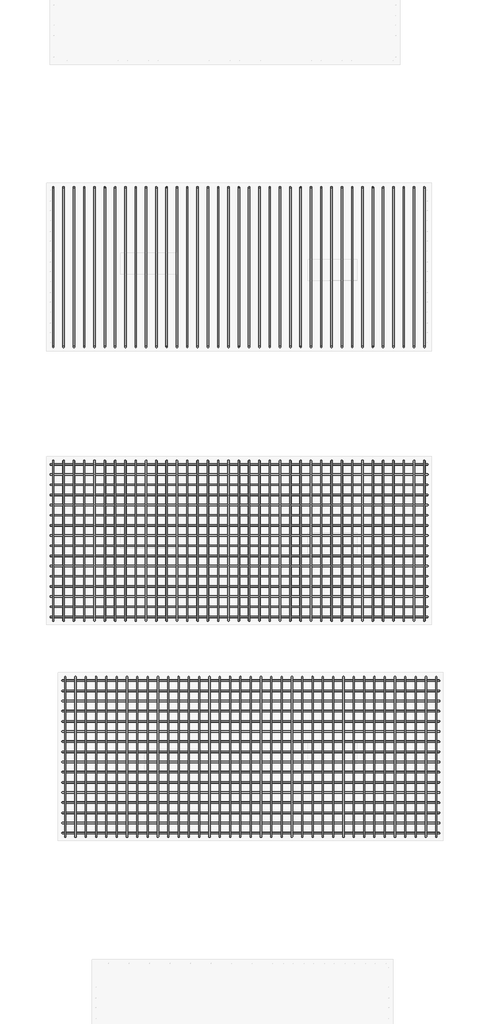
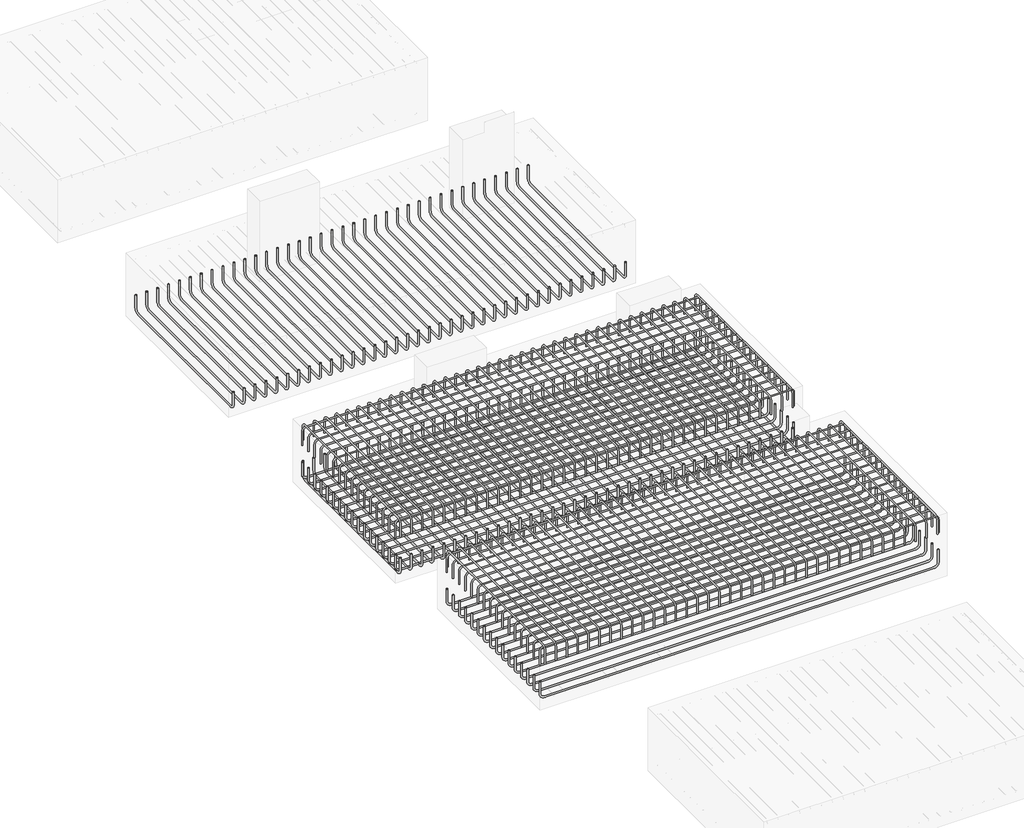
# One storey, part 5 of 21: 8 reinforcing bars.
"""IFC4 building model written with IfcOpenShell, lengths in millimetres."""

from ifc_helpers import new_model, si_unit, point, frame, origin, place, context, project, spatial, polyline, circle_curve, trimmed, segment, composite_curve, source, transform, mapped, element, save
from ifc_brep_helpers import swept_disk

model = new_model("IFC4")

# Units and contexts
model_context = context("Model", 3, world=origin())
ifc_project = project(units=[si_unit("LENGTHUNIT", "METRE", prefix="MILLI")], contexts=[model_context])

# Site, building, storey
site = spatial("IfcSite", under=ifc_project)
building = spatial("IfcBuilding", under=site)
storey = spatial("IfcBuildingStorey", under=building, Elevation=-1100.0)

# Reinforcing bars
placement = place(None, origin())
reinforcing_bar_shape = source(origin(), model_context, "Body", "SolidModel", [
    swept_disk(composite_curve([segment(polyline([(-19444.5839151, -8642.8795712, -1400.0), (-19444.5839151, -8642.8795712, -1213.4)]), True, "CONTINUOUS"), segment(trimmed(circle_curve(frame((-19444.5839151, -8587.4295712, -1213.4), z_axis=(-1.0, 0.0, 0.0), x_axis=(0.0, -55.44999999999891, 0.0)), 55.45), [point((-19444.5839151, -8642.8795712, -1213.4))], [point((-19444.5839151, -8587.4295712, -1157.95))], True, "CARTESIAN"), True, "CONTINUOUS"), segment(polyline([(-19444.5839151, -8587.4295712, -1157.95), (-19444.5839151, -6414.2295712, -1157.95)]), True, "CONTINUOUS"), segment(trimmed(circle_curve(frame((-19444.5839151, -6414.2295712, -1213.4), z_axis=(-1.0, 0.0, 0.0), x_axis=(0.0, 0.0, 55.450000000000045)), 55.45), [point((-19444.5839151, -6414.2295712, -1157.95))], [point((-19444.5839151, -6358.7795712, -1213.4))], True, "CARTESIAN"), True, "CONTINUOUS"), segment(polyline([(-19444.5839151, -6358.7795712, -1213.4), (-19444.5839151, -6358.7795712, -1400.0)]), True, "CONTINUOUS")], self_intersect=False), 7.95),
])
element("IfcReinforcingBar", 1, at=placement, inside=storey, context=model_context, shape_type="MappedRepresentation", body=[
    mapped(reinforcing_bar_shape, transform((0.0, 0.0, 0.0), x_axis=(1.0, 0.0, 0.0), y_axis=(0.0, 1.0, 0.0), z_axis=(0.0, 0.0, 1.0))),
    mapped(reinforcing_bar_shape, transform((147.2696553, 0.0, 0.0), x_axis=(1.0, 0.0, 0.0), y_axis=(0.0, 1.0, 0.0), z_axis=(0.0, 0.0, 1.0))),
    mapped(reinforcing_bar_shape, transform((294.5393106, 0.0, 0.0), x_axis=(1.0, 0.0, 0.0), y_axis=(0.0, 1.0, 0.0), z_axis=(0.0, 0.0, 1.0))),
    mapped(reinforcing_bar_shape, transform((441.8089659, 0.0, 0.0), x_axis=(1.0, 0.0, 0.0), y_axis=(0.0, 1.0, 0.0), z_axis=(0.0, 0.0, 1.0))),
    mapped(reinforcing_bar_shape, transform((589.0786213, 0.0, 0.0), x_axis=(1.0, 0.0, 0.0), y_axis=(0.0, 1.0, 0.0), z_axis=(0.0, 0.0, 1.0))),
    mapped(reinforcing_bar_shape, transform((736.3482766, 0.0, 0.0), x_axis=(1.0, 0.0, 0.0), y_axis=(0.0, 1.0, 0.0), z_axis=(0.0, 0.0, 1.0))),
    mapped(reinforcing_bar_shape, transform((883.6179319, 0.0, 0.0), x_axis=(1.0, 0.0, 0.0), y_axis=(0.0, 1.0, 0.0), z_axis=(0.0, 0.0, 1.0))),
    mapped(reinforcing_bar_shape, transform((1030.8875872, 0.0, 0.0), x_axis=(1.0, 0.0, 0.0), y_axis=(0.0, 1.0, 0.0), z_axis=(0.0, 0.0, 1.0))),
    mapped(reinforcing_bar_shape, transform((1178.1572425, 0.0, 0.0), x_axis=(1.0, 0.0, 0.0), y_axis=(0.0, 1.0, 0.0), z_axis=(0.0, 0.0, 1.0))),
    mapped(reinforcing_bar_shape, transform((1325.4268978, 0.0, 0.0), x_axis=(1.0, 0.0, 0.0), y_axis=(0.0, 1.0, 0.0), z_axis=(0.0, 0.0, 1.0))),
    mapped(reinforcing_bar_shape, transform((1472.6965532, 0.0, 0.0), x_axis=(1.0, 0.0, 0.0), y_axis=(0.0, 1.0, 0.0), z_axis=(0.0, 0.0, 1.0))),
    mapped(reinforcing_bar_shape, transform((1619.9662085, 0.0, 0.0), x_axis=(1.0, 0.0, 0.0), y_axis=(0.0, 1.0, 0.0), z_axis=(0.0, 0.0, 1.0))),
    mapped(reinforcing_bar_shape, transform((1767.2358638, 0.0, 0.0), x_axis=(1.0, 0.0, 0.0), y_axis=(0.0, 1.0, 0.0), z_axis=(0.0, 0.0, 1.0))),
    mapped(reinforcing_bar_shape, transform((1914.5055191, 0.0, 0.0), x_axis=(1.0, 0.0, 0.0), y_axis=(0.0, 1.0, 0.0), z_axis=(0.0, 0.0, 1.0))),
    mapped(reinforcing_bar_shape, transform((2061.7751744, 0.0, 0.0), x_axis=(1.0, 0.0, 0.0), y_axis=(0.0, 1.0, 0.0), z_axis=(0.0, 0.0, 1.0))),
    mapped(reinforcing_bar_shape, transform((2209.0448297, 0.0, 0.0), x_axis=(1.0, 0.0, 0.0), y_axis=(0.0, 1.0, 0.0), z_axis=(0.0, 0.0, 1.0))),
    mapped(reinforcing_bar_shape, transform((2356.314485, 0.0, 0.0), x_axis=(1.0, 0.0, 0.0), y_axis=(0.0, 1.0, 0.0), z_axis=(0.0, 0.0, 1.0))),
    mapped(reinforcing_bar_shape, transform((2503.5841404, 0.0, 0.0), x_axis=(1.0, 0.0, 0.0), y_axis=(0.0, 1.0, 0.0), z_axis=(0.0, 0.0, 1.0))),
    mapped(reinforcing_bar_shape, transform((2650.8537957, 0.0, 0.0), x_axis=(1.0, 0.0, 0.0), y_axis=(0.0, 1.0, 0.0), z_axis=(0.0, 0.0, 1.0))),
    mapped(reinforcing_bar_shape, transform((2798.123451, 0.0, 0.0), x_axis=(1.0, 0.0, 0.0), y_axis=(0.0, 1.0, 0.0), z_axis=(0.0, 0.0, 1.0))),
    mapped(reinforcing_bar_shape, transform((2945.3931063, 0.0, 0.0), x_axis=(1.0, 0.0, 0.0), y_axis=(0.0, 1.0, 0.0), z_axis=(0.0, 0.0, 1.0))),
    mapped(reinforcing_bar_shape, transform((3092.6627616, 0.0, 0.0), x_axis=(1.0, 0.0, 0.0), y_axis=(0.0, 1.0, 0.0), z_axis=(0.0, 0.0, 1.0))),
    mapped(reinforcing_bar_shape, transform((3239.9324169, 0.0, 0.0), x_axis=(1.0, 0.0, 0.0), y_axis=(0.0, 1.0, 0.0), z_axis=(0.0, 0.0, 1.0))),
    mapped(reinforcing_bar_shape, transform((3387.2020722, 0.0, 0.0), x_axis=(1.0, 0.0, 0.0), y_axis=(0.0, 1.0, 0.0), z_axis=(0.0, 0.0, 1.0))),
    mapped(reinforcing_bar_shape, transform((3534.4717276, 0.0, 0.0), x_axis=(1.0, 0.0, 0.0), y_axis=(0.0, 1.0, 0.0), z_axis=(0.0, 0.0, 1.0))),
    mapped(reinforcing_bar_shape, transform((3681.7413829, 0.0, 0.0), x_axis=(1.0, 0.0, 0.0), y_axis=(0.0, 1.0, 0.0), z_axis=(0.0, 0.0, 1.0))),
    mapped(reinforcing_bar_shape, transform((3829.0110382, 0.0, 0.0), x_axis=(1.0, 0.0, 0.0), y_axis=(0.0, 1.0, 0.0), z_axis=(0.0, 0.0, 1.0))),
    mapped(reinforcing_bar_shape, transform((3976.2806935, 0.0, 0.0), x_axis=(1.0, 0.0, 0.0), y_axis=(0.0, 1.0, 0.0), z_axis=(0.0, 0.0, 1.0))),
    mapped(reinforcing_bar_shape, transform((4123.5503488, 0.0, 0.0), x_axis=(1.0, 0.0, 0.0), y_axis=(0.0, 1.0, 0.0), z_axis=(0.0, 0.0, 1.0))),
    mapped(reinforcing_bar_shape, transform((4270.8200041, 0.0, 0.0), x_axis=(1.0, 0.0, 0.0), y_axis=(0.0, 1.0, 0.0), z_axis=(0.0, 0.0, 1.0))),
    mapped(reinforcing_bar_shape, transform((4418.0896595, 0.0, 0.0), x_axis=(1.0, 0.0, 0.0), y_axis=(0.0, 1.0, 0.0), z_axis=(0.0, 0.0, 1.0))),
    mapped(reinforcing_bar_shape, transform((4565.3593148, 0.0, 0.0), x_axis=(1.0, 0.0, 0.0), y_axis=(0.0, 1.0, 0.0), z_axis=(0.0, 0.0, 1.0))),
    mapped(reinforcing_bar_shape, transform((4712.6289701, 0.0, 0.0), x_axis=(1.0, 0.0, 0.0), y_axis=(0.0, 1.0, 0.0), z_axis=(0.0, 0.0, 1.0))),
    mapped(reinforcing_bar_shape, transform((4859.8986254, 0.0, 0.0), x_axis=(1.0, 0.0, 0.0), y_axis=(0.0, 1.0, 0.0), z_axis=(0.0, 0.0, 1.0))),
    mapped(reinforcing_bar_shape, transform((5007.1682807, 0.0, 0.0), x_axis=(1.0, 0.0, 0.0), y_axis=(0.0, 1.0, 0.0), z_axis=(0.0, 0.0, 1.0))),
    mapped(reinforcing_bar_shape, transform((5154.437936, 0.0, 0.0), x_axis=(1.0, 0.0, 0.0), y_axis=(0.0, 1.0, 0.0), z_axis=(0.0, 0.0, 1.0))),
    mapped(reinforcing_bar_shape, transform((5301.7075913, 0.0, 0.0), x_axis=(1.0, 0.0, 0.0), y_axis=(0.0, 1.0, 0.0), z_axis=(0.0, 0.0, 1.0))),
])
reinforcing_bar_2_shape = source(origin(), model_context, "Body", "SolidModel", [
    swept_disk(composite_curve([segment(polyline([(-19482.8826863, -6410.6137352, -1428.1111113), (-19482.8826863, -6410.6137352, -1241.5111113)]), True, "CONTINUOUS"), segment(trimmed(circle_curve(frame((-19427.4326863, -6410.6137352, -1241.5111113), z_axis=(0.0, 1.0, 0.0), x_axis=(-55.45000000000073, 0.0, 0.0)), 55.45), [point((-19482.8826863, -6410.6137352, -1241.5111113))], [point((-19427.4326863, -6410.6137352, -1186.0611113))], True, "CARTESIAN"), True, "CONTINUOUS"), segment(polyline([(-19427.4326863, -6410.6137352, -1186.0611113), (-14154.2326863, -6410.6137352, -1186.0611113)]), True, "CONTINUOUS"), segment(trimmed(circle_curve(frame((-14154.2326863, -6410.6137352, -1241.5111113), z_axis=(0.0, 1.0, 0.0), x_axis=(0.0, 0.0, 55.450000000000045)), 55.45), [point((-14154.2326863, -6410.6137352, -1186.0611113))], [point((-14098.7826863, -6410.6137352, -1241.5111113))], True, "CARTESIAN"), True, "CONTINUOUS"), segment(polyline([(-14098.7826863, -6410.6137352, -1241.5111113), (-14098.7826863, -6410.6137352, -1428.1111113)]), True, "CONTINUOUS")], self_intersect=False), 7.95),
])
element("IfcReinforcingBar", 2, at=placement, inside=storey, context=model_context, shape_type="MappedRepresentation", body=[
    mapped(reinforcing_bar_2_shape, transform((0.0, 0.0, 0.0), x_axis=(1.0, 0.0, 0.0), y_axis=(0.0, 1.0, 0.0), z_axis=(0.0, 0.0, 1.0))),
    mapped(reinforcing_bar_2_shape, transform((0.0, -145.2528929, 0.0), x_axis=(1.0, 0.0, 0.0), y_axis=(0.0, 1.0, 0.0), z_axis=(0.0, 0.0, 1.0))),
    mapped(reinforcing_bar_2_shape, transform((0.0, -290.5057858, 0.0), x_axis=(1.0, 0.0, 0.0), y_axis=(0.0, 1.0, 0.0), z_axis=(0.0, 0.0, 1.0))),
    mapped(reinforcing_bar_2_shape, transform((0.0, -435.7586787, 0.0), x_axis=(1.0, 0.0, 0.0), y_axis=(0.0, 1.0, 0.0), z_axis=(0.0, 0.0, 1.0))),
    mapped(reinforcing_bar_2_shape, transform((0.0, -581.0115716, 0.0), x_axis=(1.0, 0.0, 0.0), y_axis=(0.0, 1.0, 0.0), z_axis=(0.0, 0.0, 1.0))),
    mapped(reinforcing_bar_2_shape, transform((0.0, -726.2644645, 0.0), x_axis=(1.0, 0.0, 0.0), y_axis=(0.0, 1.0, 0.0), z_axis=(0.0, 0.0, 1.0))),
    mapped(reinforcing_bar_2_shape, transform((0.0, -871.5173574, 0.0), x_axis=(1.0, 0.0, 0.0), y_axis=(0.0, 1.0, 0.0), z_axis=(0.0, 0.0, 1.0))),
    mapped(reinforcing_bar_2_shape, transform((0.0, -1016.7702503, 0.0), x_axis=(1.0, 0.0, 0.0), y_axis=(0.0, 1.0, 0.0), z_axis=(0.0, 0.0, 1.0))),
    mapped(reinforcing_bar_2_shape, transform((0.0, -1162.0231432, 0.0), x_axis=(1.0, 0.0, 0.0), y_axis=(0.0, 1.0, 0.0), z_axis=(0.0, 0.0, 1.0))),
    mapped(reinforcing_bar_2_shape, transform((0.0, -1307.276036, 0.0), x_axis=(1.0, 0.0, 0.0), y_axis=(0.0, 1.0, 0.0), z_axis=(0.0, 0.0, 1.0))),
    mapped(reinforcing_bar_2_shape, transform((0.0, -1452.5289289, 0.0), x_axis=(1.0, 0.0, 0.0), y_axis=(0.0, 1.0, 0.0), z_axis=(0.0, 0.0, 1.0))),
    mapped(reinforcing_bar_2_shape, transform((0.0, -1597.7818218, 0.0), x_axis=(1.0, 0.0, 0.0), y_axis=(0.0, 1.0, 0.0), z_axis=(0.0, 0.0, 1.0))),
    mapped(reinforcing_bar_2_shape, transform((0.0, -1743.0347147, 0.0), x_axis=(1.0, 0.0, 0.0), y_axis=(0.0, 1.0, 0.0), z_axis=(0.0, 0.0, 1.0))),
    mapped(reinforcing_bar_2_shape, transform((0.0, -1888.2876076, 0.0), x_axis=(1.0, 0.0, 0.0), y_axis=(0.0, 1.0, 0.0), z_axis=(0.0, 0.0, 1.0))),
    mapped(reinforcing_bar_2_shape, transform((0.0, -2033.5405005, 0.0), x_axis=(1.0, 0.0, 0.0), y_axis=(0.0, 1.0, 0.0), z_axis=(0.0, 0.0, 1.0))),
    mapped(reinforcing_bar_2_shape, transform((0.0, -2178.7933934, 0.0), x_axis=(1.0, 0.0, 0.0), y_axis=(0.0, 1.0, 0.0), z_axis=(0.0, 0.0, 1.0))),
])
reinforcing_bar_3_shape = source(origin(), model_context, "Body", "SolidModel", [
    swept_disk(composite_curve([segment(polyline([(-19480.8326863, -8589.4071286, -1669.8442859), (-19480.8326863, -8589.4071286, -1852.3442859)]), True, "CONTINUOUS"), segment(trimmed(circle_curve(frame((-19423.3326863, -8589.4071286, -1852.3442859), z_axis=(0.0, -1.0, 0.0), x_axis=(-57.5, 0.0, 0.0)), 57.5), [point((-19480.8326863, -8589.4071286, -1852.3442859))], [point((-19423.3326863, -8589.4071286, -1909.8442859))], True, "CARTESIAN"), True, "CONTINUOUS"), segment(polyline([(-19423.3326863, -8589.4071286, -1909.8442859), (-14158.3326863, -8589.4071286, -1909.8442859)]), True, "CONTINUOUS"), segment(trimmed(circle_curve(frame((-14158.3326863, -8589.4071286, -1852.3442859), z_axis=(0.0, -1.0, 0.0), x_axis=(0.0, 0.0, -57.5)), 57.5), [point((-14158.3326863, -8589.4071286, -1909.8442859))], [point((-14100.8326863, -8589.4071286, -1852.3442859))], True, "CARTESIAN"), True, "CONTINUOUS"), segment(polyline([(-14100.8326863, -8589.4071286, -1852.3442859), (-14100.8326863, -8589.4071286, -1669.8442859)]), True, "CONTINUOUS")], self_intersect=False), 10.0),
])
element("IfcReinforcingBar", 3, at=placement, inside=storey, context=model_context, shape_type="MappedRepresentation", body=[
    mapped(reinforcing_bar_3_shape, transform((0.0, 0.0, 0.0), x_axis=(1.0, 0.0, 0.0), y_axis=(0.0, 1.0, 0.0), z_axis=(0.0, 0.0, 1.0))),
    mapped(reinforcing_bar_3_shape, transform((0.0, 145.2528929, 0.0), x_axis=(1.0, 0.0, 0.0), y_axis=(0.0, 1.0, 0.0), z_axis=(0.0, 0.0, 1.0))),
    mapped(reinforcing_bar_3_shape, transform((0.0, 290.5057858, 0.0), x_axis=(1.0, 0.0, 0.0), y_axis=(0.0, 1.0, 0.0), z_axis=(0.0, 0.0, 1.0))),
    mapped(reinforcing_bar_3_shape, transform((0.0, 435.7586787, 0.0), x_axis=(1.0, 0.0, 0.0), y_axis=(0.0, 1.0, 0.0), z_axis=(0.0, 0.0, 1.0))),
    mapped(reinforcing_bar_3_shape, transform((0.0, 581.0115716, 0.0), x_axis=(1.0, 0.0, 0.0), y_axis=(0.0, 1.0, 0.0), z_axis=(0.0, 0.0, 1.0))),
    mapped(reinforcing_bar_3_shape, transform((0.0, 726.2644645, 0.0), x_axis=(1.0, 0.0, 0.0), y_axis=(0.0, 1.0, 0.0), z_axis=(0.0, 0.0, 1.0))),
    mapped(reinforcing_bar_3_shape, transform((0.0, 871.5173574, 0.0), x_axis=(1.0, 0.0, 0.0), y_axis=(0.0, 1.0, 0.0), z_axis=(0.0, 0.0, 1.0))),
    mapped(reinforcing_bar_3_shape, transform((0.0, 1016.7702503, 0.0), x_axis=(1.0, 0.0, 0.0), y_axis=(0.0, 1.0, 0.0), z_axis=(0.0, 0.0, 1.0))),
    mapped(reinforcing_bar_3_shape, transform((0.0, 1162.0231432, 0.0), x_axis=(1.0, 0.0, 0.0), y_axis=(0.0, 1.0, 0.0), z_axis=(0.0, 0.0, 1.0))),
    mapped(reinforcing_bar_3_shape, transform((0.0, 1307.276036, 0.0), x_axis=(1.0, 0.0, 0.0), y_axis=(0.0, 1.0, 0.0), z_axis=(0.0, 0.0, 1.0))),
    mapped(reinforcing_bar_3_shape, transform((0.0, 1452.5289289, 0.0), x_axis=(1.0, 0.0, 0.0), y_axis=(0.0, 1.0, 0.0), z_axis=(0.0, 0.0, 1.0))),
    mapped(reinforcing_bar_3_shape, transform((0.0, 1597.7818218, 0.0), x_axis=(1.0, 0.0, 0.0), y_axis=(0.0, 1.0, 0.0), z_axis=(0.0, 0.0, 1.0))),
    mapped(reinforcing_bar_3_shape, transform((0.0, 1743.0347147, 0.0), x_axis=(1.0, 0.0, 0.0), y_axis=(0.0, 1.0, 0.0), z_axis=(0.0, 0.0, 1.0))),
    mapped(reinforcing_bar_3_shape, transform((0.0, 1888.2876076, 0.0), x_axis=(1.0, 0.0, 0.0), y_axis=(0.0, 1.0, 0.0), z_axis=(0.0, 0.0, 1.0))),
    mapped(reinforcing_bar_3_shape, transform((0.0, 2033.5405005, 0.0), x_axis=(1.0, 0.0, 0.0), y_axis=(0.0, 1.0, 0.0), z_axis=(0.0, 0.0, 1.0))),
    mapped(reinforcing_bar_3_shape, transform((0.0, 2178.7933934, 0.0), x_axis=(1.0, 0.0, 0.0), y_axis=(0.0, 1.0, 0.0), z_axis=(0.0, 0.0, 1.0))),
])
reinforcing_bar_4_shape = source(origin(), model_context, "Body", "SolidModel", [
    swept_disk(composite_curve([segment(polyline([(-19614.5839151, -3270.8295712, -1700.0), (-19614.5839151, -3270.8295712, -1882.5)]), True, "CONTINUOUS"), segment(trimmed(circle_curve(frame((-19614.5839151, -3328.3295712, -1882.5), z_axis=(-1.0, 0.0, 0.0), x_axis=(0.0, 57.5, 0.0)), 57.5), [point((-19614.5839151, -3270.8295712, -1882.5))], [point((-19614.5839151, -3328.3295712, -1940.0))], True, "CARTESIAN"), True, "CONTINUOUS"), segment(polyline([(-19614.5839151, -3328.3295712, -1940.0), (-19614.5839151, -5493.3295712, -1940.0)]), True, "CONTINUOUS"), segment(trimmed(circle_curve(frame((-19614.5839151, -5493.3295712, -1882.5), z_axis=(-1.0, 0.0, 0.0), x_axis=(0.0, 0.0, -57.5)), 57.5), [point((-19614.5839151, -5493.3295712, -1940.0))], [point((-19614.5839151, -5550.8295712, -1882.5))], True, "CARTESIAN"), True, "CONTINUOUS"), segment(polyline([(-19614.5839151, -5550.8295712, -1882.5), (-19614.5839151, -5550.8295712, -1700.0)]), True, "CONTINUOUS")], self_intersect=False), 10.0),
])
element("IfcReinforcingBar", 4, at=placement, inside=storey, context=model_context, shape_type="MappedRepresentation", body=[
    mapped(reinforcing_bar_4_shape, transform((0.0, 0.0, 0.0), x_axis=(1.0, 0.0, 0.0), y_axis=(0.0, 1.0, 0.0), z_axis=(0.0, 0.0, 1.0))),
    mapped(reinforcing_bar_4_shape, transform((147.2696553, 0.0, 0.0), x_axis=(1.0, 0.0, 0.0), y_axis=(0.0, 1.0, 0.0), z_axis=(0.0, 0.0, 1.0))),
    mapped(reinforcing_bar_4_shape, transform((294.5393106, 0.0, 0.0), x_axis=(1.0, 0.0, 0.0), y_axis=(0.0, 1.0, 0.0), z_axis=(0.0, 0.0, 1.0))),
    mapped(reinforcing_bar_4_shape, transform((441.8089659, 0.0, 0.0), x_axis=(1.0, 0.0, 0.0), y_axis=(0.0, 1.0, 0.0), z_axis=(0.0, 0.0, 1.0))),
    mapped(reinforcing_bar_4_shape, transform((589.0786213, 0.0, 0.0), x_axis=(1.0, 0.0, 0.0), y_axis=(0.0, 1.0, 0.0), z_axis=(0.0, 0.0, 1.0))),
    mapped(reinforcing_bar_4_shape, transform((736.3482766, 0.0, 0.0), x_axis=(1.0, 0.0, 0.0), y_axis=(0.0, 1.0, 0.0), z_axis=(0.0, 0.0, 1.0))),
    mapped(reinforcing_bar_4_shape, transform((883.6179319, 0.0, 0.0), x_axis=(1.0, 0.0, 0.0), y_axis=(0.0, 1.0, 0.0), z_axis=(0.0, 0.0, 1.0))),
    mapped(reinforcing_bar_4_shape, transform((1030.8875872, 0.0, 0.0), x_axis=(1.0, 0.0, 0.0), y_axis=(0.0, 1.0, 0.0), z_axis=(0.0, 0.0, 1.0))),
    mapped(reinforcing_bar_4_shape, transform((1178.1572425, 0.0, 0.0), x_axis=(1.0, 0.0, 0.0), y_axis=(0.0, 1.0, 0.0), z_axis=(0.0, 0.0, 1.0))),
    mapped(reinforcing_bar_4_shape, transform((1325.4268978, 0.0, 0.0), x_axis=(1.0, 0.0, 0.0), y_axis=(0.0, 1.0, 0.0), z_axis=(0.0, 0.0, 1.0))),
    mapped(reinforcing_bar_4_shape, transform((1472.6965532, 0.0, 0.0), x_axis=(1.0, 0.0, 0.0), y_axis=(0.0, 1.0, 0.0), z_axis=(0.0, 0.0, 1.0))),
    mapped(reinforcing_bar_4_shape, transform((1619.9662085, 0.0, 0.0), x_axis=(1.0, 0.0, 0.0), y_axis=(0.0, 1.0, 0.0), z_axis=(0.0, 0.0, 1.0))),
    mapped(reinforcing_bar_4_shape, transform((1767.2358638, 0.0, 0.0), x_axis=(1.0, 0.0, 0.0), y_axis=(0.0, 1.0, 0.0), z_axis=(0.0, 0.0, 1.0))),
    mapped(reinforcing_bar_4_shape, transform((1914.5055191, 0.0, 0.0), x_axis=(1.0, 0.0, 0.0), y_axis=(0.0, 1.0, 0.0), z_axis=(0.0, 0.0, 1.0))),
    mapped(reinforcing_bar_4_shape, transform((2061.7751744, 0.0, 0.0), x_axis=(1.0, 0.0, 0.0), y_axis=(0.0, 1.0, 0.0), z_axis=(0.0, 0.0, 1.0))),
    mapped(reinforcing_bar_4_shape, transform((2209.0448297, 0.0, 0.0), x_axis=(1.0, 0.0, 0.0), y_axis=(0.0, 1.0, 0.0), z_axis=(0.0, 0.0, 1.0))),
    mapped(reinforcing_bar_4_shape, transform((2356.314485, 0.0, 0.0), x_axis=(1.0, 0.0, 0.0), y_axis=(0.0, 1.0, 0.0), z_axis=(0.0, 0.0, 1.0))),
    mapped(reinforcing_bar_4_shape, transform((2503.5841404, 0.0, 0.0), x_axis=(1.0, 0.0, 0.0), y_axis=(0.0, 1.0, 0.0), z_axis=(0.0, 0.0, 1.0))),
    mapped(reinforcing_bar_4_shape, transform((2650.8537957, 0.0, 0.0), x_axis=(1.0, 0.0, 0.0), y_axis=(0.0, 1.0, 0.0), z_axis=(0.0, 0.0, 1.0))),
    mapped(reinforcing_bar_4_shape, transform((2798.123451, 0.0, 0.0), x_axis=(1.0, 0.0, 0.0), y_axis=(0.0, 1.0, 0.0), z_axis=(0.0, 0.0, 1.0))),
    mapped(reinforcing_bar_4_shape, transform((2945.3931063, 0.0, 0.0), x_axis=(1.0, 0.0, 0.0), y_axis=(0.0, 1.0, 0.0), z_axis=(0.0, 0.0, 1.0))),
    mapped(reinforcing_bar_4_shape, transform((3092.6627616, 0.0, 0.0), x_axis=(1.0, 0.0, 0.0), y_axis=(0.0, 1.0, 0.0), z_axis=(0.0, 0.0, 1.0))),
    mapped(reinforcing_bar_4_shape, transform((3239.9324169, 0.0, 0.0), x_axis=(1.0, 0.0, 0.0), y_axis=(0.0, 1.0, 0.0), z_axis=(0.0, 0.0, 1.0))),
    mapped(reinforcing_bar_4_shape, transform((3387.2020722, 0.0, 0.0), x_axis=(1.0, 0.0, 0.0), y_axis=(0.0, 1.0, 0.0), z_axis=(0.0, 0.0, 1.0))),
    mapped(reinforcing_bar_4_shape, transform((3534.4717276, 0.0, 0.0), x_axis=(1.0, 0.0, 0.0), y_axis=(0.0, 1.0, 0.0), z_axis=(0.0, 0.0, 1.0))),
    mapped(reinforcing_bar_4_shape, transform((3681.7413829, 0.0, 0.0), x_axis=(1.0, 0.0, 0.0), y_axis=(0.0, 1.0, 0.0), z_axis=(0.0, 0.0, 1.0))),
    mapped(reinforcing_bar_4_shape, transform((3829.0110382, 0.0, 0.0), x_axis=(1.0, 0.0, 0.0), y_axis=(0.0, 1.0, 0.0), z_axis=(0.0, 0.0, 1.0))),
    mapped(reinforcing_bar_4_shape, transform((3976.2806935, 0.0, 0.0), x_axis=(1.0, 0.0, 0.0), y_axis=(0.0, 1.0, 0.0), z_axis=(0.0, 0.0, 1.0))),
    mapped(reinforcing_bar_4_shape, transform((4123.5503488, 0.0, 0.0), x_axis=(1.0, 0.0, 0.0), y_axis=(0.0, 1.0, 0.0), z_axis=(0.0, 0.0, 1.0))),
    mapped(reinforcing_bar_4_shape, transform((4270.8200041, 0.0, 0.0), x_axis=(1.0, 0.0, 0.0), y_axis=(0.0, 1.0, 0.0), z_axis=(0.0, 0.0, 1.0))),
    mapped(reinforcing_bar_4_shape, transform((4418.0896595, 0.0, 0.0), x_axis=(1.0, 0.0, 0.0), y_axis=(0.0, 1.0, 0.0), z_axis=(0.0, 0.0, 1.0))),
    mapped(reinforcing_bar_4_shape, transform((4565.3593148, 0.0, 0.0), x_axis=(1.0, 0.0, 0.0), y_axis=(0.0, 1.0, 0.0), z_axis=(0.0, 0.0, 1.0))),
    mapped(reinforcing_bar_4_shape, transform((4712.6289701, 0.0, 0.0), x_axis=(1.0, 0.0, 0.0), y_axis=(0.0, 1.0, 0.0), z_axis=(0.0, 0.0, 1.0))),
    mapped(reinforcing_bar_4_shape, transform((4859.8986254, 0.0, 0.0), x_axis=(1.0, 0.0, 0.0), y_axis=(0.0, 1.0, 0.0), z_axis=(0.0, 0.0, 1.0))),
    mapped(reinforcing_bar_4_shape, transform((5007.1682807, 0.0, 0.0), x_axis=(1.0, 0.0, 0.0), y_axis=(0.0, 1.0, 0.0), z_axis=(0.0, 0.0, 1.0))),
    mapped(reinforcing_bar_4_shape, transform((5154.437936, 0.0, 0.0), x_axis=(1.0, 0.0, 0.0), y_axis=(0.0, 1.0, 0.0), z_axis=(0.0, 0.0, 1.0))),
    mapped(reinforcing_bar_4_shape, transform((5301.7075913, 0.0, 0.0), x_axis=(1.0, 0.0, 0.0), y_axis=(0.0, 1.0, 0.0), z_axis=(0.0, 0.0, 1.0))),
])
reinforcing_bar_5_shape = source(origin(), model_context, "Body", "SolidModel", [
    swept_disk(composite_curve([segment(polyline([(-19614.5839151, -5552.8795712, -1400.0), (-19614.5839151, -5552.8795712, -1213.4)]), True, "CONTINUOUS"), segment(trimmed(circle_curve(frame((-19614.5839151, -5497.4295712, -1213.4), z_axis=(-1.0, 0.0, 0.0), x_axis=(0.0, -55.44999999999982, 0.0)), 55.45), [point((-19614.5839151, -5552.8795712, -1213.4))], [point((-19614.5839151, -5497.4295712, -1157.95))], True, "CARTESIAN"), True, "CONTINUOUS"), segment(polyline([(-19614.5839151, -5497.4295712, -1157.95), (-19614.5839151, -3324.2295712, -1157.95)]), True, "CONTINUOUS"), segment(trimmed(circle_curve(frame((-19614.5839151, -3324.2295712, -1213.4), z_axis=(-1.0, 0.0, 0.0), x_axis=(0.0, 0.0, 55.450000000000045)), 55.45), [point((-19614.5839151, -3324.2295712, -1157.95))], [point((-19614.5839151, -3268.7795712, -1213.4))], True, "CARTESIAN"), True, "CONTINUOUS"), segment(polyline([(-19614.5839151, -3268.7795712, -1213.4), (-19614.5839151, -3268.7795712, -1400.0)]), True, "CONTINUOUS")], self_intersect=False), 7.95),
])
element("IfcReinforcingBar", 5, at=placement, inside=storey, context=model_context, shape_type="MappedRepresentation", body=[
    mapped(reinforcing_bar_5_shape, transform((0.0, 0.0, 0.0), x_axis=(1.0, 0.0, 0.0), y_axis=(0.0, 1.0, 0.0), z_axis=(0.0, 0.0, 1.0))),
    mapped(reinforcing_bar_5_shape, transform((147.2696553, 0.0, 0.0), x_axis=(1.0, 0.0, 0.0), y_axis=(0.0, 1.0, 0.0), z_axis=(0.0, 0.0, 1.0))),
    mapped(reinforcing_bar_5_shape, transform((294.5393106, 0.0, 0.0), x_axis=(1.0, 0.0, 0.0), y_axis=(0.0, 1.0, 0.0), z_axis=(0.0, 0.0, 1.0))),
    mapped(reinforcing_bar_5_shape, transform((441.8089659, 0.0, 0.0), x_axis=(1.0, 0.0, 0.0), y_axis=(0.0, 1.0, 0.0), z_axis=(0.0, 0.0, 1.0))),
    mapped(reinforcing_bar_5_shape, transform((589.0786213, 0.0, 0.0), x_axis=(1.0, 0.0, 0.0), y_axis=(0.0, 1.0, 0.0), z_axis=(0.0, 0.0, 1.0))),
    mapped(reinforcing_bar_5_shape, transform((736.3482766, 0.0, 0.0), x_axis=(1.0, 0.0, 0.0), y_axis=(0.0, 1.0, 0.0), z_axis=(0.0, 0.0, 1.0))),
    mapped(reinforcing_bar_5_shape, transform((883.6179319, 0.0, 0.0), x_axis=(1.0, 0.0, 0.0), y_axis=(0.0, 1.0, 0.0), z_axis=(0.0, 0.0, 1.0))),
    mapped(reinforcing_bar_5_shape, transform((1030.8875872, 0.0, 0.0), x_axis=(1.0, 0.0, 0.0), y_axis=(0.0, 1.0, 0.0), z_axis=(0.0, 0.0, 1.0))),
    mapped(reinforcing_bar_5_shape, transform((1178.1572425, 0.0, 0.0), x_axis=(1.0, 0.0, 0.0), y_axis=(0.0, 1.0, 0.0), z_axis=(0.0, 0.0, 1.0))),
    mapped(reinforcing_bar_5_shape, transform((1325.4268978, 0.0, 0.0), x_axis=(1.0, 0.0, 0.0), y_axis=(0.0, 1.0, 0.0), z_axis=(0.0, 0.0, 1.0))),
    mapped(reinforcing_bar_5_shape, transform((1472.6965532, 0.0, 0.0), x_axis=(1.0, 0.0, 0.0), y_axis=(0.0, 1.0, 0.0), z_axis=(0.0, 0.0, 1.0))),
    mapped(reinforcing_bar_5_shape, transform((1619.9662085, 0.0, 0.0), x_axis=(1.0, 0.0, 0.0), y_axis=(0.0, 1.0, 0.0), z_axis=(0.0, 0.0, 1.0))),
    mapped(reinforcing_bar_5_shape, transform((1767.2358638, 0.0, 0.0), x_axis=(1.0, 0.0, 0.0), y_axis=(0.0, 1.0, 0.0), z_axis=(0.0, 0.0, 1.0))),
    mapped(reinforcing_bar_5_shape, transform((1914.5055191, 0.0, 0.0), x_axis=(1.0, 0.0, 0.0), y_axis=(0.0, 1.0, 0.0), z_axis=(0.0, 0.0, 1.0))),
    mapped(reinforcing_bar_5_shape, transform((2061.7751744, 0.0, 0.0), x_axis=(1.0, 0.0, 0.0), y_axis=(0.0, 1.0, 0.0), z_axis=(0.0, 0.0, 1.0))),
    mapped(reinforcing_bar_5_shape, transform((2209.0448297, 0.0, 0.0), x_axis=(1.0, 0.0, 0.0), y_axis=(0.0, 1.0, 0.0), z_axis=(0.0, 0.0, 1.0))),
    mapped(reinforcing_bar_5_shape, transform((2356.314485, 0.0, 0.0), x_axis=(1.0, 0.0, 0.0), y_axis=(0.0, 1.0, 0.0), z_axis=(0.0, 0.0, 1.0))),
    mapped(reinforcing_bar_5_shape, transform((2503.5841404, 0.0, 0.0), x_axis=(1.0, 0.0, 0.0), y_axis=(0.0, 1.0, 0.0), z_axis=(0.0, 0.0, 1.0))),
    mapped(reinforcing_bar_5_shape, transform((2650.8537957, 0.0, 0.0), x_axis=(1.0, 0.0, 0.0), y_axis=(0.0, 1.0, 0.0), z_axis=(0.0, 0.0, 1.0))),
    mapped(reinforcing_bar_5_shape, transform((2798.123451, 0.0, 0.0), x_axis=(1.0, 0.0, 0.0), y_axis=(0.0, 1.0, 0.0), z_axis=(0.0, 0.0, 1.0))),
    mapped(reinforcing_bar_5_shape, transform((2945.3931063, 0.0, 0.0), x_axis=(1.0, 0.0, 0.0), y_axis=(0.0, 1.0, 0.0), z_axis=(0.0, 0.0, 1.0))),
    mapped(reinforcing_bar_5_shape, transform((3092.6627616, 0.0, 0.0), x_axis=(1.0, 0.0, 0.0), y_axis=(0.0, 1.0, 0.0), z_axis=(0.0, 0.0, 1.0))),
    mapped(reinforcing_bar_5_shape, transform((3239.9324169, 0.0, 0.0), x_axis=(1.0, 0.0, 0.0), y_axis=(0.0, 1.0, 0.0), z_axis=(0.0, 0.0, 1.0))),
    mapped(reinforcing_bar_5_shape, transform((3387.2020722, 0.0, 0.0), x_axis=(1.0, 0.0, 0.0), y_axis=(0.0, 1.0, 0.0), z_axis=(0.0, 0.0, 1.0))),
    mapped(reinforcing_bar_5_shape, transform((3534.4717276, 0.0, 0.0), x_axis=(1.0, 0.0, 0.0), y_axis=(0.0, 1.0, 0.0), z_axis=(0.0, 0.0, 1.0))),
    mapped(reinforcing_bar_5_shape, transform((3681.7413829, 0.0, 0.0), x_axis=(1.0, 0.0, 0.0), y_axis=(0.0, 1.0, 0.0), z_axis=(0.0, 0.0, 1.0))),
    mapped(reinforcing_bar_5_shape, transform((3829.0110382, 0.0, 0.0), x_axis=(1.0, 0.0, 0.0), y_axis=(0.0, 1.0, 0.0), z_axis=(0.0, 0.0, 1.0))),
    mapped(reinforcing_bar_5_shape, transform((3976.2806935, 0.0, 0.0), x_axis=(1.0, 0.0, 0.0), y_axis=(0.0, 1.0, 0.0), z_axis=(0.0, 0.0, 1.0))),
    mapped(reinforcing_bar_5_shape, transform((4123.5503488, 0.0, 0.0), x_axis=(1.0, 0.0, 0.0), y_axis=(0.0, 1.0, 0.0), z_axis=(0.0, 0.0, 1.0))),
    mapped(reinforcing_bar_5_shape, transform((4270.8200041, 0.0, 0.0), x_axis=(1.0, 0.0, 0.0), y_axis=(0.0, 1.0, 0.0), z_axis=(0.0, 0.0, 1.0))),
    mapped(reinforcing_bar_5_shape, transform((4418.0896595, 0.0, 0.0), x_axis=(1.0, 0.0, 0.0), y_axis=(0.0, 1.0, 0.0), z_axis=(0.0, 0.0, 1.0))),
    mapped(reinforcing_bar_5_shape, transform((4565.3593148, 0.0, 0.0), x_axis=(1.0, 0.0, 0.0), y_axis=(0.0, 1.0, 0.0), z_axis=(0.0, 0.0, 1.0))),
    mapped(reinforcing_bar_5_shape, transform((4712.6289701, 0.0, 0.0), x_axis=(1.0, 0.0, 0.0), y_axis=(0.0, 1.0, 0.0), z_axis=(0.0, 0.0, 1.0))),
    mapped(reinforcing_bar_5_shape, transform((4859.8986254, 0.0, 0.0), x_axis=(1.0, 0.0, 0.0), y_axis=(0.0, 1.0, 0.0), z_axis=(0.0, 0.0, 1.0))),
    mapped(reinforcing_bar_5_shape, transform((5007.1682807, 0.0, 0.0), x_axis=(1.0, 0.0, 0.0), y_axis=(0.0, 1.0, 0.0), z_axis=(0.0, 0.0, 1.0))),
    mapped(reinforcing_bar_5_shape, transform((5154.437936, 0.0, 0.0), x_axis=(1.0, 0.0, 0.0), y_axis=(0.0, 1.0, 0.0), z_axis=(0.0, 0.0, 1.0))),
    mapped(reinforcing_bar_5_shape, transform((5301.7075913, 0.0, 0.0), x_axis=(1.0, 0.0, 0.0), y_axis=(0.0, 1.0, 0.0), z_axis=(0.0, 0.0, 1.0))),
])
reinforcing_bar_6_shape = source(origin(), model_context, "Body", "SolidModel", [
    swept_disk(composite_curve([segment(polyline([(-19652.8826863, -3320.6137352, -1428.1111113), (-19652.8826863, -3320.6137352, -1241.5111113)]), True, "CONTINUOUS"), segment(trimmed(circle_curve(frame((-19597.4326863, -3320.6137352, -1241.5111113), z_axis=(0.0, 1.0, 0.0), x_axis=(-55.45000000000073, 0.0, 0.0)), 55.45), [point((-19652.8826863, -3320.6137352, -1241.5111113))], [point((-19597.4326863, -3320.6137352, -1186.0611113))], True, "CARTESIAN"), True, "CONTINUOUS"), segment(polyline([(-19597.4326863, -3320.6137352, -1186.0611113), (-14324.2326863, -3320.6137352, -1186.0611113)]), True, "CONTINUOUS"), segment(trimmed(circle_curve(frame((-14324.2326863, -3320.6137352, -1241.5111113), z_axis=(0.0, 1.0, 0.0), x_axis=(0.0, 0.0, 55.450000000000045)), 55.45), [point((-14324.2326863, -3320.6137352, -1186.0611113))], [point((-14268.7826863, -3320.6137352, -1241.5111113))], True, "CARTESIAN"), True, "CONTINUOUS"), segment(polyline([(-14268.7826863, -3320.6137352, -1241.5111113), (-14268.7826863, -3320.6137352, -1428.1111113)]), True, "CONTINUOUS")], self_intersect=False), 7.95),
])
element("IfcReinforcingBar", 6, at=placement, inside=storey, context=model_context, shape_type="MappedRepresentation", body=[
    mapped(reinforcing_bar_6_shape, transform((0.0, 0.0, 0.0), x_axis=(1.0, 0.0, 0.0), y_axis=(0.0, 1.0, 0.0), z_axis=(0.0, 0.0, 1.0))),
    mapped(reinforcing_bar_6_shape, transform((0.0, -145.2528929, 0.0), x_axis=(1.0, 0.0, 0.0), y_axis=(0.0, 1.0, 0.0), z_axis=(0.0, 0.0, 1.0))),
    mapped(reinforcing_bar_6_shape, transform((0.0, -290.5057858, 0.0), x_axis=(1.0, 0.0, 0.0), y_axis=(0.0, 1.0, 0.0), z_axis=(0.0, 0.0, 1.0))),
    mapped(reinforcing_bar_6_shape, transform((0.0, -435.7586787, 0.0), x_axis=(1.0, 0.0, 0.0), y_axis=(0.0, 1.0, 0.0), z_axis=(0.0, 0.0, 1.0))),
    mapped(reinforcing_bar_6_shape, transform((0.0, -581.0115716, 0.0), x_axis=(1.0, 0.0, 0.0), y_axis=(0.0, 1.0, 0.0), z_axis=(0.0, 0.0, 1.0))),
    mapped(reinforcing_bar_6_shape, transform((0.0, -726.2644645, 0.0), x_axis=(1.0, 0.0, 0.0), y_axis=(0.0, 1.0, 0.0), z_axis=(0.0, 0.0, 1.0))),
    mapped(reinforcing_bar_6_shape, transform((0.0, -871.5173574, 0.0), x_axis=(1.0, 0.0, 0.0), y_axis=(0.0, 1.0, 0.0), z_axis=(0.0, 0.0, 1.0))),
    mapped(reinforcing_bar_6_shape, transform((0.0, -1016.7702503, 0.0), x_axis=(1.0, 0.0, 0.0), y_axis=(0.0, 1.0, 0.0), z_axis=(0.0, 0.0, 1.0))),
    mapped(reinforcing_bar_6_shape, transform((0.0, -1162.0231432, 0.0), x_axis=(1.0, 0.0, 0.0), y_axis=(0.0, 1.0, 0.0), z_axis=(0.0, 0.0, 1.0))),
    mapped(reinforcing_bar_6_shape, transform((0.0, -1307.276036, 0.0), x_axis=(1.0, 0.0, 0.0), y_axis=(0.0, 1.0, 0.0), z_axis=(0.0, 0.0, 1.0))),
    mapped(reinforcing_bar_6_shape, transform((0.0, -1452.5289289, 0.0), x_axis=(1.0, 0.0, 0.0), y_axis=(0.0, 1.0, 0.0), z_axis=(0.0, 0.0, 1.0))),
    mapped(reinforcing_bar_6_shape, transform((0.0, -1597.7818218, 0.0), x_axis=(1.0, 0.0, 0.0), y_axis=(0.0, 1.0, 0.0), z_axis=(0.0, 0.0, 1.0))),
    mapped(reinforcing_bar_6_shape, transform((0.0, -1743.0347147, 0.0), x_axis=(1.0, 0.0, 0.0), y_axis=(0.0, 1.0, 0.0), z_axis=(0.0, 0.0, 1.0))),
    mapped(reinforcing_bar_6_shape, transform((0.0, -1888.2876076, 0.0), x_axis=(1.0, 0.0, 0.0), y_axis=(0.0, 1.0, 0.0), z_axis=(0.0, 0.0, 1.0))),
    mapped(reinforcing_bar_6_shape, transform((0.0, -2033.5405005, 0.0), x_axis=(1.0, 0.0, 0.0), y_axis=(0.0, 1.0, 0.0), z_axis=(0.0, 0.0, 1.0))),
    mapped(reinforcing_bar_6_shape, transform((0.0, -2178.7933934, 0.0), x_axis=(1.0, 0.0, 0.0), y_axis=(0.0, 1.0, 0.0), z_axis=(0.0, 0.0, 1.0))),
])
reinforcing_bar_7_shape = source(origin(), model_context, "Body", "SolidModel", [
    swept_disk(composite_curve([segment(polyline([(-19650.8326863, -5499.4071286, -1669.8442859), (-19650.8326863, -5499.4071286, -1852.3442859)]), True, "CONTINUOUS"), segment(trimmed(circle_curve(frame((-19593.3326863, -5499.4071286, -1852.3442859), z_axis=(0.0, -1.0, 0.0), x_axis=(-57.5, 0.0, 0.0)), 57.5), [point((-19650.8326863, -5499.4071286, -1852.3442859))], [point((-19593.3326863, -5499.4071286, -1909.8442859))], True, "CARTESIAN"), True, "CONTINUOUS"), segment(polyline([(-19593.3326863, -5499.4071286, -1909.8442859), (-14328.3326863, -5499.4071286, -1909.8442859)]), True, "CONTINUOUS"), segment(trimmed(circle_curve(frame((-14328.3326863, -5499.4071286, -1852.3442859), z_axis=(0.0, -1.0, 0.0), x_axis=(0.0, 0.0, -57.5)), 57.5), [point((-14328.3326863, -5499.4071286, -1909.8442859))], [point((-14270.8326863, -5499.4071286, -1852.3442859))], True, "CARTESIAN"), True, "CONTINUOUS"), segment(polyline([(-14270.8326863, -5499.4071286, -1852.3442859), (-14270.8326863, -5499.4071286, -1669.8442859)]), True, "CONTINUOUS")], self_intersect=False), 10.0),
])
element("IfcReinforcingBar", 7, at=placement, inside=storey, context=model_context, shape_type="MappedRepresentation", body=[
    mapped(reinforcing_bar_7_shape, transform((0.0, 0.0, 0.0), x_axis=(1.0, 0.0, 0.0), y_axis=(0.0, 1.0, 0.0), z_axis=(0.0, 0.0, 1.0))),
    mapped(reinforcing_bar_7_shape, transform((0.0, 145.2528929, 0.0), x_axis=(1.0, 0.0, 0.0), y_axis=(0.0, 1.0, 0.0), z_axis=(0.0, 0.0, 1.0))),
    mapped(reinforcing_bar_7_shape, transform((0.0, 290.5057858, 0.0), x_axis=(1.0, 0.0, 0.0), y_axis=(0.0, 1.0, 0.0), z_axis=(0.0, 0.0, 1.0))),
    mapped(reinforcing_bar_7_shape, transform((0.0, 435.7586787, 0.0), x_axis=(1.0, 0.0, 0.0), y_axis=(0.0, 1.0, 0.0), z_axis=(0.0, 0.0, 1.0))),
    mapped(reinforcing_bar_7_shape, transform((0.0, 581.0115716, 0.0), x_axis=(1.0, 0.0, 0.0), y_axis=(0.0, 1.0, 0.0), z_axis=(0.0, 0.0, 1.0))),
    mapped(reinforcing_bar_7_shape, transform((0.0, 726.2644645, 0.0), x_axis=(1.0, 0.0, 0.0), y_axis=(0.0, 1.0, 0.0), z_axis=(0.0, 0.0, 1.0))),
    mapped(reinforcing_bar_7_shape, transform((0.0, 871.5173574, 0.0), x_axis=(1.0, 0.0, 0.0), y_axis=(0.0, 1.0, 0.0), z_axis=(0.0, 0.0, 1.0))),
    mapped(reinforcing_bar_7_shape, transform((0.0, 1016.7702503, 0.0), x_axis=(1.0, 0.0, 0.0), y_axis=(0.0, 1.0, 0.0), z_axis=(0.0, 0.0, 1.0))),
    mapped(reinforcing_bar_7_shape, transform((0.0, 1162.0231432, 0.0), x_axis=(1.0, 0.0, 0.0), y_axis=(0.0, 1.0, 0.0), z_axis=(0.0, 0.0, 1.0))),
    mapped(reinforcing_bar_7_shape, transform((0.0, 1307.276036, 0.0), x_axis=(1.0, 0.0, 0.0), y_axis=(0.0, 1.0, 0.0), z_axis=(0.0, 0.0, 1.0))),
    mapped(reinforcing_bar_7_shape, transform((0.0, 1452.5289289, 0.0), x_axis=(1.0, 0.0, 0.0), y_axis=(0.0, 1.0, 0.0), z_axis=(0.0, 0.0, 1.0))),
    mapped(reinforcing_bar_7_shape, transform((0.0, 1597.7818218, 0.0), x_axis=(1.0, 0.0, 0.0), y_axis=(0.0, 1.0, 0.0), z_axis=(0.0, 0.0, 1.0))),
    mapped(reinforcing_bar_7_shape, transform((0.0, 1743.0347147, 0.0), x_axis=(1.0, 0.0, 0.0), y_axis=(0.0, 1.0, 0.0), z_axis=(0.0, 0.0, 1.0))),
    mapped(reinforcing_bar_7_shape, transform((0.0, 1888.2876076, 0.0), x_axis=(1.0, 0.0, 0.0), y_axis=(0.0, 1.0, 0.0), z_axis=(0.0, 0.0, 1.0))),
    mapped(reinforcing_bar_7_shape, transform((0.0, 2033.5405005, 0.0), x_axis=(1.0, 0.0, 0.0), y_axis=(0.0, 1.0, 0.0), z_axis=(0.0, 0.0, 1.0))),
    mapped(reinforcing_bar_7_shape, transform((0.0, 2178.7933934, 0.0), x_axis=(1.0, 0.0, 0.0), y_axis=(0.0, 1.0, 0.0), z_axis=(0.0, 0.0, 1.0))),
])
reinforcing_bar_8_shape = source(origin(), model_context, "Body", "SolidModel", [
    swept_disk(composite_curve([segment(polyline([(-19614.5839151, 639.1704288, -1700.0), (-19614.5839151, 639.1704288, -1882.5)]), True, "CONTINUOUS"), segment(trimmed(circle_curve(frame((-19614.5839151, 581.6704288, -1882.5), z_axis=(-1.0, 0.0, 0.0), x_axis=(0.0, 57.5, 0.0)), 57.5), [point((-19614.5839151, 639.1704288, -1882.5))], [point((-19614.5839151, 581.6704288, -1940.0))], True, "CARTESIAN"), True, "CONTINUOUS"), segment(polyline([(-19614.5839151, 581.6704288, -1940.0), (-19614.5839151, -1583.3295712, -1940.0)]), True, "CONTINUOUS"), segment(trimmed(circle_curve(frame((-19614.5839151, -1583.3295712, -1882.5), z_axis=(-1.0, 0.0, 0.0), x_axis=(0.0, 0.0, -57.5)), 57.5), [point((-19614.5839151, -1583.3295712, -1940.0))], [point((-19614.5839151, -1640.8295712, -1882.5))], True, "CARTESIAN"), True, "CONTINUOUS"), segment(polyline([(-19614.5839151, -1640.8295712, -1882.5), (-19614.5839151, -1640.8295712, -1700.0)]), True, "CONTINUOUS")], self_intersect=False), 10.0),
])
element("IfcReinforcingBar", 8, at=placement, inside=storey, context=model_context, shape_type="MappedRepresentation", body=[
    mapped(reinforcing_bar_8_shape, transform((0.0, 0.0, 0.0), x_axis=(1.0, 0.0, 0.0), y_axis=(0.0, 1.0, 0.0), z_axis=(0.0, 0.0, 1.0))),
    mapped(reinforcing_bar_8_shape, transform((147.2696553, 0.0, 0.0), x_axis=(1.0, 0.0, 0.0), y_axis=(0.0, 1.0, 0.0), z_axis=(0.0, 0.0, 1.0))),
    mapped(reinforcing_bar_8_shape, transform((294.5393106, 0.0, 0.0), x_axis=(1.0, 0.0, 0.0), y_axis=(0.0, 1.0, 0.0), z_axis=(0.0, 0.0, 1.0))),
    mapped(reinforcing_bar_8_shape, transform((441.8089659, 0.0, 0.0), x_axis=(1.0, 0.0, 0.0), y_axis=(0.0, 1.0, 0.0), z_axis=(0.0, 0.0, 1.0))),
    mapped(reinforcing_bar_8_shape, transform((589.0786213, 0.0, 0.0), x_axis=(1.0, 0.0, 0.0), y_axis=(0.0, 1.0, 0.0), z_axis=(0.0, 0.0, 1.0))),
    mapped(reinforcing_bar_8_shape, transform((736.3482766, 0.0, 0.0), x_axis=(1.0, 0.0, 0.0), y_axis=(0.0, 1.0, 0.0), z_axis=(0.0, 0.0, 1.0))),
    mapped(reinforcing_bar_8_shape, transform((883.6179319, 0.0, 0.0), x_axis=(1.0, 0.0, 0.0), y_axis=(0.0, 1.0, 0.0), z_axis=(0.0, 0.0, 1.0))),
    mapped(reinforcing_bar_8_shape, transform((1030.8875872, 0.0, 0.0), x_axis=(1.0, 0.0, 0.0), y_axis=(0.0, 1.0, 0.0), z_axis=(0.0, 0.0, 1.0))),
    mapped(reinforcing_bar_8_shape, transform((1178.1572425, 0.0, 0.0), x_axis=(1.0, 0.0, 0.0), y_axis=(0.0, 1.0, 0.0), z_axis=(0.0, 0.0, 1.0))),
    mapped(reinforcing_bar_8_shape, transform((1325.4268978, 0.0, 0.0), x_axis=(1.0, 0.0, 0.0), y_axis=(0.0, 1.0, 0.0), z_axis=(0.0, 0.0, 1.0))),
    mapped(reinforcing_bar_8_shape, transform((1472.6965532, 0.0, 0.0), x_axis=(1.0, 0.0, 0.0), y_axis=(0.0, 1.0, 0.0), z_axis=(0.0, 0.0, 1.0))),
    mapped(reinforcing_bar_8_shape, transform((1619.9662085, 0.0, 0.0), x_axis=(1.0, 0.0, 0.0), y_axis=(0.0, 1.0, 0.0), z_axis=(0.0, 0.0, 1.0))),
    mapped(reinforcing_bar_8_shape, transform((1767.2358638, 0.0, 0.0), x_axis=(1.0, 0.0, 0.0), y_axis=(0.0, 1.0, 0.0), z_axis=(0.0, 0.0, 1.0))),
    mapped(reinforcing_bar_8_shape, transform((1914.5055191, 0.0, 0.0), x_axis=(1.0, 0.0, 0.0), y_axis=(0.0, 1.0, 0.0), z_axis=(0.0, 0.0, 1.0))),
    mapped(reinforcing_bar_8_shape, transform((2061.7751744, 0.0, 0.0), x_axis=(1.0, 0.0, 0.0), y_axis=(0.0, 1.0, 0.0), z_axis=(0.0, 0.0, 1.0))),
    mapped(reinforcing_bar_8_shape, transform((2209.0448297, 0.0, 0.0), x_axis=(1.0, 0.0, 0.0), y_axis=(0.0, 1.0, 0.0), z_axis=(0.0, 0.0, 1.0))),
    mapped(reinforcing_bar_8_shape, transform((2356.314485, 0.0, 0.0), x_axis=(1.0, 0.0, 0.0), y_axis=(0.0, 1.0, 0.0), z_axis=(0.0, 0.0, 1.0))),
    mapped(reinforcing_bar_8_shape, transform((2503.5841404, 0.0, 0.0), x_axis=(1.0, 0.0, 0.0), y_axis=(0.0, 1.0, 0.0), z_axis=(0.0, 0.0, 1.0))),
    mapped(reinforcing_bar_8_shape, transform((2650.8537957, 0.0, 0.0), x_axis=(1.0, 0.0, 0.0), y_axis=(0.0, 1.0, 0.0), z_axis=(0.0, 0.0, 1.0))),
    mapped(reinforcing_bar_8_shape, transform((2798.123451, 0.0, 0.0), x_axis=(1.0, 0.0, 0.0), y_axis=(0.0, 1.0, 0.0), z_axis=(0.0, 0.0, 1.0))),
    mapped(reinforcing_bar_8_shape, transform((2945.3931063, 0.0, 0.0), x_axis=(1.0, 0.0, 0.0), y_axis=(0.0, 1.0, 0.0), z_axis=(0.0, 0.0, 1.0))),
    mapped(reinforcing_bar_8_shape, transform((3092.6627616, 0.0, 0.0), x_axis=(1.0, 0.0, 0.0), y_axis=(0.0, 1.0, 0.0), z_axis=(0.0, 0.0, 1.0))),
    mapped(reinforcing_bar_8_shape, transform((3239.9324169, 0.0, 0.0), x_axis=(1.0, 0.0, 0.0), y_axis=(0.0, 1.0, 0.0), z_axis=(0.0, 0.0, 1.0))),
    mapped(reinforcing_bar_8_shape, transform((3387.2020722, 0.0, 0.0), x_axis=(1.0, 0.0, 0.0), y_axis=(0.0, 1.0, 0.0), z_axis=(0.0, 0.0, 1.0))),
    mapped(reinforcing_bar_8_shape, transform((3534.4717276, 0.0, 0.0), x_axis=(1.0, 0.0, 0.0), y_axis=(0.0, 1.0, 0.0), z_axis=(0.0, 0.0, 1.0))),
    mapped(reinforcing_bar_8_shape, transform((3681.7413829, 0.0, 0.0), x_axis=(1.0, 0.0, 0.0), y_axis=(0.0, 1.0, 0.0), z_axis=(0.0, 0.0, 1.0))),
    mapped(reinforcing_bar_8_shape, transform((3829.0110382, 0.0, 0.0), x_axis=(1.0, 0.0, 0.0), y_axis=(0.0, 1.0, 0.0), z_axis=(0.0, 0.0, 1.0))),
    mapped(reinforcing_bar_8_shape, transform((3976.2806935, 0.0, 0.0), x_axis=(1.0, 0.0, 0.0), y_axis=(0.0, 1.0, 0.0), z_axis=(0.0, 0.0, 1.0))),
    mapped(reinforcing_bar_8_shape, transform((4123.5503488, 0.0, 0.0), x_axis=(1.0, 0.0, 0.0), y_axis=(0.0, 1.0, 0.0), z_axis=(0.0, 0.0, 1.0))),
    mapped(reinforcing_bar_8_shape, transform((4270.8200041, 0.0, 0.0), x_axis=(1.0, 0.0, 0.0), y_axis=(0.0, 1.0, 0.0), z_axis=(0.0, 0.0, 1.0))),
    mapped(reinforcing_bar_8_shape, transform((4418.0896595, 0.0, 0.0), x_axis=(1.0, 0.0, 0.0), y_axis=(0.0, 1.0, 0.0), z_axis=(0.0, 0.0, 1.0))),
    mapped(reinforcing_bar_8_shape, transform((4565.3593148, 0.0, 0.0), x_axis=(1.0, 0.0, 0.0), y_axis=(0.0, 1.0, 0.0), z_axis=(0.0, 0.0, 1.0))),
    mapped(reinforcing_bar_8_shape, transform((4712.6289701, 0.0, 0.0), x_axis=(1.0, 0.0, 0.0), y_axis=(0.0, 1.0, 0.0), z_axis=(0.0, 0.0, 1.0))),
    mapped(reinforcing_bar_8_shape, transform((4859.8986254, 0.0, 0.0), x_axis=(1.0, 0.0, 0.0), y_axis=(0.0, 1.0, 0.0), z_axis=(0.0, 0.0, 1.0))),
    mapped(reinforcing_bar_8_shape, transform((5007.1682807, 0.0, 0.0), x_axis=(1.0, 0.0, 0.0), y_axis=(0.0, 1.0, 0.0), z_axis=(0.0, 0.0, 1.0))),
    mapped(reinforcing_bar_8_shape, transform((5154.437936, 0.0, 0.0), x_axis=(1.0, 0.0, 0.0), y_axis=(0.0, 1.0, 0.0), z_axis=(0.0, 0.0, 1.0))),
    mapped(reinforcing_bar_8_shape, transform((5301.7075913, 0.0, 0.0), x_axis=(1.0, 0.0, 0.0), y_axis=(0.0, 1.0, 0.0), z_axis=(0.0, 0.0, 1.0))),
])

save(model, "model.ifc")

# Revit data of these elements
# Elements 1, 2, 3, 4, 5, 6, 7, 8 (IfcReinforcingBar)
#   Phase Created = New Construction
